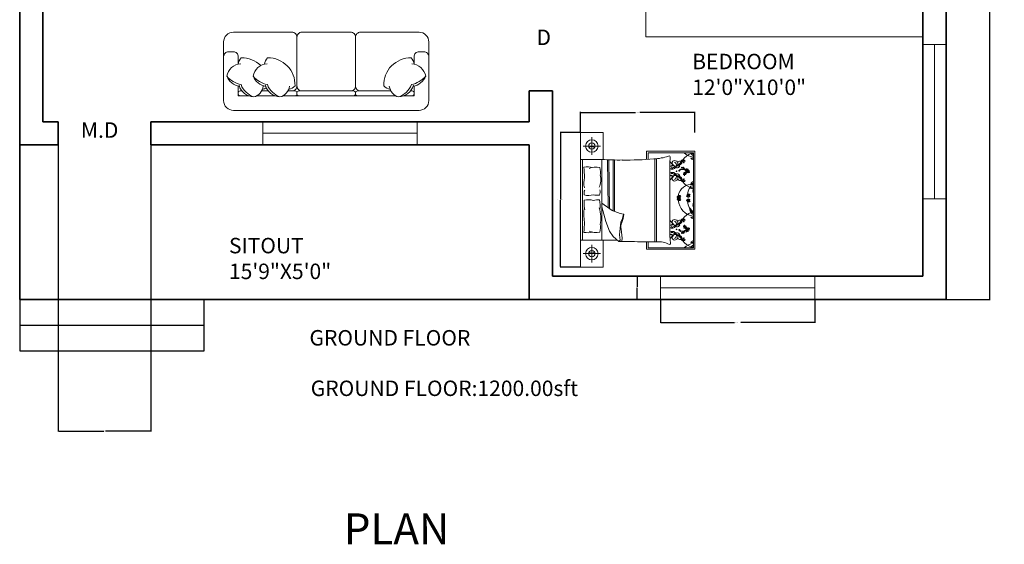
# Model space of a CAD drawing. Units: inches. Extents: x -43 to 1296, y -568 to 542.
# Tile 1 of 14: x 29 to 411, y -568 to -365. Entities that reach past the tile are written whole.
import ezdxf

# ---------------------------------------------------------------- set-up
doc = ezdxf.new("R2010")
doc.units = ezdxf.units.IN
doc.header["$MEASUREMENT"] = 0
for name, color, linetype, lineweight in [('A-ANNO-DIMS', 2, 'Continuous', 18), ('A-ANNO-TEXT', 7, 'Continuous', 18), ('A-AREA-IDEN', 7, 'Continuous', 18), ('A-FLOR-CASE', 9, 'Continuous', 18), ('A-FLOR-STRS', 7, 'Continuous', 25), ('A-FURN', 8, 'Continuous', 13), ('A-GLAZ', 6, 'Continuous', 18), ('A-WALL', 7, 'Continuous', 35)]:
    doc.layers.add(name, color=color, linetype=linetype, lineweight=lineweight)
doc.styles.get("Standard").update_dxf_attribs({"font": 'arial.ttf'})
doc.dimstyles.get("Standard").update_dxf_attribs({"dimtxt": 0.18, "dimasz": 0.18, "dimexe": 0.18, "dimexo": 0.0625, "dimgap": 0.09, "dimtad": 0, "dimtih": 1, "dimtoh": 1, "dimdec": 0, "dimzin": 0, "dimdsep": 46, "dimlunit": 3, "dimtxsty": 'Standard', "dimcen": 0.09, "dimadec": 0, "dimazin": 0, "dimtfac": 1, "dimtdec": 0, "dimtofl": 0, "dimtmove": 0, "dimatfit": 3, "dimfxl": 1, "dimtolj": 1, "dimtzin": 0, "dimarcsym": 0})

# ---------------------------------------------------------------- blocks, each defined once
blk = doc.blocks.new('*D2')
at = {"layer": 'A-ANNO-DIMS', "color": 0, "lineweight": -2, "transparency": 16777216}
for p, q in [((388.91, 6.66), (405.97, 6.66)), ((405.79, 6.48), (405.79, -230.19)), ((405.79, -473.16), (405.79, -236.49)), ((388.91, -473.34), (405.97, -473.34))]:
    blk.add_line(p, q, dxfattribs=at)
at = {"layer": 'A-ANNO-DIMS', "color": 0, "transparency": 16777216}
for points in [[(405.76, 6.48), (405.82, 6.48), (405.79, 6.66)], [(405.76, -473.16), (405.82, -473.16), (405.79, -473.34)]]:
    blk.add_solid(points, dxfattribs=at)
at = {"layer": 'Defpoints', "color": 0, "transparency": 16777216}
for p in [(388.84, 6.66), (388.84, -473.34), (405.79, -473.34)]:
    blk.add_point(p, dxfattribs=at)
at = {"layer": 'A-ANNO-DIMS', "color": 0, "transparency": 16777216, "insert": (405.79, -233.34), "char_height": 6, "attachment_point": 5}
blk.add_mtext("\\A1;40'", dxfattribs=at)
blk = doc.blocks.new('BED-SUITE-52')
for p, q in [((0, 0), (0, 52.23)), ((4.35, 43.59), (4.35, 50.42)), ((7.76, 47), (0.94, 47)), ((25.6, 42.07), (25.6, 44.97)), ((25.6, 44.97), (44.41, 44.97)), ((26.21, 44.36), (26.21, 42.06)), ((43.81, 44.36), (26.21, 44.36)), ((43.81, 7.5), (43.81, 44.36)), ((44.41, 44.97), (44.41, 6.89)), ((0.67, 41.78), (0.67, 10.45)), ((8.25, 10.45), (8.25, 41.78)), ((10.42, 41.64), (10.68, 23.05)), ((10.96, 41.62), (11.23, 22.66)), ((12.6, 41.59), (12.68, 21.76)), ((13.14, 41.6), (13.22, 21.56)), ((28.86, 42.02), (28.86, 9.84)), ((29.51, 42.07), (29.51, 9.84)), ((38.51, 39.22), (37.92, 39.33)), ((34.64, 36.72), (34.64, 15.51)), ((38.51, 35.57), (37.92, 35.45)), ((8.25, 24.79), (12.24, 21.93)), ((9.81, 17.7), (8.25, 23.4)), ((12.24, 21.93), (15.3, 20.77)), ((15.3, 20.77), (16.68, 20.56)), ((16.68, 20.56), (16.25, 18.86)), ((11.18, 13.89), (9.81, 17.7)), ((15.62, 17.49), (15.3, 15.16)), ((16.25, 18.86), (15.62, 17.49)), ((38.51, 16.3), (37.92, 16.41)), ((12.66, 11.88), (11.18, 13.89)), ((14.88, 9.98), (12.66, 11.88)), ((15.3, 15.16), (15.09, 12.52)), ((15.09, 12.52), (15.3, 10.4)), ((38.51, 12.65), (37.92, 12.53)), ((0, 10.45), (14.33, 10.45)), ((4.35, 8.64), (4.35, 1.81)), ((15.3, 10.4), (14.88, 9.98)), ((25.6, 6.89), (25.6, 9.85)), ((26.21, 9.85), (26.21, 7.5)), ((7.76, 5.22), (0.94, 5.22)), ((44.41, 6.89), (25.6, 6.89)), ((26.21, 7.5), (43.81, 7.5))]:
    blk.add_line(p, q)
for points in [[(0, 41.78), (8.7, 41.78), (8.7, 52.23), (0, 52.23)], [(4.35, 47), (3.3, 46.39)], [(4.35, 47), (5.41, 46.39)], [(8.7, 10.45), (8.7, 0), (0, 0)], [(4.35, 5.22), (3.3, 5.83)], [(4.35, 5.22), (5.41, 5.83)]]:
    blk.add_lwpolyline(points)
for points in [[(28.45, 42, 0.056112), (31.32, 42.38, 0.095341), (34.09, 43.12)], [(1.3, 38.78, -0.074897), (4.71, 38.72, 0.472817)], [(4.9, 28.1, -0.14099), (1.42, 27.99, -0.235245)], [(4.9, 25.87, 0.14099), (1.42, 25.97, 0.235245)], [(1.3, 13.45, 0.074897), (4.71, 13.51, -0.472817)], [(19.66, 9.87, 0.001242), (29.57, 9.84, -0.127202), (34.51, 8.8)]]:
    blk.add_lwpolyline(points, format="xyb")
for centre, radius in [((4.35, 47), 2.44), ((4.35, 47), 1.22), ((40.41, 36.2), 0.133), ((41.81, 37.07), 0.133), ((40.41, 15.66), 0.133), ((41.81, 14.79), 0.133), ((4.35, 5.22), 2.44), ((4.35, 5.22), 1.22)]:
    blk.add_circle(centre, radius)
for centre, radius, start, end in [((34.35, 42.72), 0.476, 336.5219, 123.8264), ((85.43, 38.32), 50.82, 175.2402, 181.8035), ((45.4, 37.77), 6.82, 111.4092, 145.6135), ((44.73, 49.44), 6.82, 228.1144, 262.255), ((45.64, 46.02), 3.32, 209.8884, 236.5383), ((44.87, 44.16), 2.77, 221.0454, 247.4453), ((43.38, 51.75), 9.44, 266.3481, 272.5919), ((46.26, 47.22), 4.14, 223.5186, 233.6964), ((-495.72, 9.99), 497.85, 2.8502, 3.3148), ((6.08, 32.13), 6.73, 78.2417, 114.8684), ((0.69, 36.92), 7, 348.9631, 14.8961), ((14.64, 135.41), 93.84, 266.1, 270.9282), ((18.05, 163.97), 122.41, 269.1145, 274.8735), ((35.22, 38.66), 0.629, 196.6343, 225.5483), ((35.03, 41.34), 2.16, 259.249, 301.1782), ((35.22, 38.66), 0.629, 127.675, 162.5814), ((38.32, 42.79), 3.95, 203.6453, 236.3329), ((35.59, 39.66), 1.66, 240.8249, 340.7178), ((35.09, 38.92), 0.781, 246.1646, 318.4347), ((35.97, 37.49), 2.01, 85.2696, 124.215), ((35.89, 39.91), 1.5, 240.0851, 262.564), ((36.42, 40.49), 0.882, 88.9462, 185.5144), ((37.07, 40.76), 1.57, 193.079, 274.7067), ((36.48, 37.7), 1.07, 74.8529, 138.4347), ((37.39, 39.86), 1.3, 196.8663, 330.0915), ((36.55, 40.12), 1.25, 7.1143, 95.0551), ((36.07, 39.63), 1.21, 338.5779, 68.4181), ((36.84, 39.04), 0.324, 254.8529, 12.6959), ((35.97, 37.49), 2.01, 53.6555, 57.2989), ((36.27, 40.34), 1.52, 305.9599, 357.6409), ((37.03, 41.99), 2.8, 273.4924, 303.7117), ((36.83, 41.97), 2.47, 288.2955, 328.7386), ((38.56, 40.41), 0.784, 19.1312, 189.736), ((38.32, 40.6), 0.979, 285.6955, 4.031), ((39.62, 39.55), 1.04, 128.4175, 173.8338), ((39.41, 40.57), 0.48, 126.7319, 206.0245), ((39.64, 41.08), 0.565, 76.272, 177.0484), ((38.78, 42.23), 1.16, 284.7031, 328.6173), ((39.25, 38.55), 0.103, 125.0752, 284.7644), ((39.41, 38.59), 0.222, 127.3642, 168.4363), ((39.24, 38.77), 0.32, 277.4968, 341.2737), ((40.4, 40.75), 1.08, 125.7657, 194.5347), ((35.12, 42.66), 4.77, 332.8176, 347.4827), ((39.49, 38.62), 0.127, 88.1325, 178.8919), ((39.75, 38.49), 0.275, 136.3462, 189.6513), ((39.62, 38.78), 0.133, 183.2768, 356.7232), ((39.59, 38.46), 0.115, 189.6513, 312.3208), ((40.03, 38.54), 0.435, 164.2829, 186.9148), ((39.52, 38.54), 0.218, 312.3208, 40.2111), ((39.98, 38.78), 0.309, 201.6382, 274.947), ((39.57, 38.36), 0.404, 42.3896, 66.5724), ((43.64, 41.56), 4.96, 217.9541, 226.8459), ((39.94, 40.89), 0.756, 20.9613, 102.2885), ((40.34, 41.64), 0.57, 181.7131, 301.5367), ((38.48, 40.49), 1.72, 2.0648, 41.1598), ((39.52, 41.13), 0.558, 316.2238, 62.3173), ((39.84, 40.8), 0.0445, 20.2667, 316.2271), ((39.86, 38.6), 0.22, 10.9597, 52.2379), ((40, 38.58), 0.102, 274.947, 37.5263), ((40.07, 40.56), 0.0411, 52.0591, 168.5166), ((40.11, 40.55), 0.0847, 168.5166, 2.0648), ((40.65, 38.13), 0.274, 115.5379, 168.6744), ((39.72, 38.52), 0.825, 329.344, 349.7412), ((39.06, 38.33), 1.47, 352.8698, 1.6736), ((10.44, 32.58), 9.18, 166.3427, 191.1841), ((1.21, 33.9), 6.65, 333.8761, 16.1746), ((35.22, 36.13), 0.629, 134.4517, 156.7144), ((35.22, 36.13), 0.629, 203.2856, 232.325), ((35.03, 33.45), 2.16, 58.8218, 100.2867), ((38.32, 32), 3.95, 123.6671, 158.5059), ((35.59, 35.12), 1.66, 19.2822, 119.1751), ((35.09, 35.86), 0.781, 41.5653, 113.8354), ((35.97, 37.29), 2.01, 235.785, 274.7304), ((35.89, 34.87), 1.5, 97.436, 119.9149), ((37.07, 34.03), 1.57, 85.2933, 166.921), ((36.48, 37.09), 1.07, 221.5653, 285.1471), ((37.39, 34.92), 1.3, 29.9085, 163.1337), ((36.55, 34.66), 1.25, 264.9449, 352.8857), ((36.07, 35.15), 1.21, 291.5819, 21.4221), ((36.84, 35.74), 0.324, 347.3041, 105.1471), ((35.97, 37.29), 2.01, 302.7011, 306.3445), ((37.27, 37.25), 0.164, 169.5864, 349.5616), ((36.27, 34.44), 1.52, 2.3591, 54.0401), ((37.03, 32.8), 2.8, 56.2883, 86.5076), ((37.33, 37.24), 0.101, 349.5616, 167.2949), ((36.83, 32.82), 2.47, 31.2614, 71.7045), ((38.56, 34.37), 0.784, 170.264, 340.8688), ((39.96, 33.62), 4.33, 110.1059, 116.9968), ((38.51, 37.19), 0.274, 129.5056, 182.6421), ((37.73, 37.82), 0.825, 308.4388, 328.836), ((37.58, 38.49), 1.47, 296.5064, 305.3102), ((37.57, 37.74), 0.839, 336.3901, 344.4871), ((38.48, 37.52), 0.106, 83.9457, 185.6216), ((38.06, 37.62), 0.438, 328.836, 0.8141), ((38.28, 37.49), 0.251, 306.5232, 32.4668), ((38.58, 37.69), 0.106, 112.5583, 214.2343), ((38.51, 37.88), 0.251, 265.7131, 351.6568), ((38.29, 38.02), 0.438, 297.3659, 329.344), ((37.96, 38.39), 0.839, 313.6929, 321.7899), ((39.62, 35.24), 1.04, 186.1662, 231.5825), ((38.32, 34.18), 0.979, 355.969, 74.3045), ((38.89, 37.82), 0.274, 115.5379, 168.6744), ((37.96, 38.21), 0.825, 329.344, 349.7412), ((39.96, 33.62), 4.33, 86.1723, 106.4158), ((37.3, 38.02), 1.47, 352.8698, 1.6736), ((40.04, 35.98), 0.103, 125.0752, 284.7644), ((40.2, 36.02), 0.222, 93.635, 168.4363), ((40.21, 37.22), 0.606, 253.6301, 325.4631), ((40.38, 36.38), 0.429, 82.0748, 142.6895), ((40.33, 36.97), 0.441, 228.342, 274.9894), ((40.17, 36.37), 0.13, 138.2946, 276.2474), ((40.03, 36.19), 0.32, 277.4968, 341.2737), ((40.22, 36.35), 0.181, 358.5719, 143.8954), ((40.28, 36.04), 0.127, 88.1325, 178.8919), ((40.33, 36.49), 0.183, 208.8493, 269.9355), ((40.17, 36.45), 0.209, 274.2123, 318.1587), ((40.34, 38), 0.106, 112.5583, 214.2343), ((40.27, 38.19), 0.251, 265.7131, 351.6568), ((40.05, 38.33), 0.438, 297.3659, 329.344), ((40.07, 35.78), 2.17, 60.7959, 85.244), ((35.46, 32.66), 7.14, 37.8256, 47.7588), ((40.54, 35.91), 0.275, 136.3462, 189.6513), ((40.38, 35.88), 0.115, 189.6513, 312.3208), ((39.72, 38.7), 0.839, 313.6929, 321.7899), ((42.95, 35.55), 2.6, 175.2415, 182.8929), ((40.34, 36.89), 0.369, 273.8774, 357.1501), ((40.82, 35.96), 0.435, 164.2829, 186.9148), ((40.81, 36.24), 0.419, 121.9501, 165.2442), ((40.49, 37.15), 0.357, 262.0748, 308.2393), ((40.31, 35.96), 0.218, 312.3208, 40.2111), ((40.77, 36.2), 0.309, 201.6382, 274.947), ((40.52, 36.4), 0.0881, 262.868, 7.094), ((40.36, 35.78), 0.404, 42.3896, 66.5724), ((40.51, 36.47), 0.262, 278.5614, 22.5914), ((40.65, 36.02), 0.22, 10.9597, 118.7804), ((42.95, 35.55), 2.6, 156.1523, 156.9499), ((40.66, 36.48), 0.132, 44.3732, 121.9501), ((41.06, 36.79), 0.369, 181.4625, 249.4747), ((42.95, 35.55), 2.6, 130.182, 149.456), ((41, 37.08), 0.357, 215.1128, 261.2773), ((41.29, 37.06), 0.606, 197.889, 269.722), ((40.79, 36), 0.102, 274.947, 37.5263), ((41.1, 36.85), 0.441, 248.3627, 295.0101), ((40.88, 36.3), 0.429, 20.6625, 81.2773), ((41.13, 38.04), 0.148, 33.0979, 123.1364), ((37.86, 35.94), 3.89, 31.1156, 34.8118), ((40.91, 37.78), 0.402, 2.3172, 70.5201), ((41.52, 37.04), 0.429, 139.3812, 199.9959), ((40.72, 37.35), 0.606, 310.9365, 22.7695), ((41, 37.31), 0.441, 285.6484, 332.2957), ((41.25, 37.68), 0.116, 135.7354, 318.1297), ((41.05, 37.87), 0.154, 315.7354, 31.1156), ((40.92, 37.55), 0.357, 319.3812, 5.5456), ((41.33, 37.68), 0.116, 68.2452, 250.6395), ((41.07, 37.83), 0.346, 352.6008, 57.1845), ((42.3, 35.5), 2.32, 111.7087, 116.2181), ((41.4, 37.91), 0.346, 252.8042, 349.6943), ((41.07, 37.29), 0.369, 331.1838, 51.6792), ((40.07, 35.78), 2.17, 47.5083, 55.9967), ((41.44, 36.85), 0.103, 125.0752, 284.7644), ((41.43, 37.93), 0.154, 248.2452, 323.6254), ((41.6, 36.89), 0.222, 93.635, 168.4363), ((41.57, 37.24), 0.13, 138.2946, 276.2474), ((41.3, 38.03), 0.402, 291.7087, 3.0299), ((41.43, 37.06), 0.32, 277.4968, 341.2737), ((41.62, 37.22), 0.181, 358.5719, 143.8954), ((38.43, 40.15), 3.89, 323.6254, 327.3216), ((41.68, 36.91), 0.127, 88.1325, 178.8919), ((41.73, 37.36), 0.183, 208.8493, 269.9355), ((41.57, 37.32), 0.209, 274.2123, 318.1587), ((41.94, 36.78), 0.275, 136.3462, 189.6513), ((41.78, 36.75), 0.115, 189.6513, 312.3208), ((41.61, 37.93), 0.148, 325.6077, 55.6462), ((42.22, 36.83), 0.435, 164.2829, 186.9148), ((42.21, 37.11), 0.419, 121.9501, 165.2442), ((41.71, 36.83), 0.218, 312.3208, 40.2111), ((42.17, 37.07), 0.309, 201.6382, 274.947), ((41.92, 37.27), 0.0881, 262.868, 7.094), ((41.76, 36.65), 0.404, 42.3896, 66.5724), ((41.91, 37.34), 0.262, 278.5614, 22.5914), ((42.06, 36.89), 0.22, 10.9597, 118.7804), ((42.06, 37.35), 0.132, 44.3732, 121.9501), ((42.19, 36.87), 0.102, 274.947, 37.5263), ((36.42, 34.3), 0.882, 174.4856, 271.0538), ((43.15, 26.86), 5.28, 82.8636, 171.8197), ((39.41, 34.21), 0.48, 153.9755, 233.2681), ((39.64, 33.71), 0.565, 182.9516, 283.728), ((38.78, 32.55), 1.16, 31.3827, 75.2969), ((40.4, 34.03), 1.08, 165.4653, 234.2343), ((35.12, 32.13), 4.77, 12.5173, 27.1824), ((38.48, 34.29), 1.72, 318.8402, 357.9352), ((39.52, 33.65), 0.558, 297.6827, 43.7762), ((40.34, 33.14), 0.57, 58.4633, 178.2869), ((39.94, 33.9), 0.756, 257.7115, 339.0387), ((45.4, 37.01), 6.82, 214.3865, 248.5908), ((39.86, 33.99), 0.0738, 43.7762, 339.7183), ((40.11, 34.24), 0.0847, 357.9352, 191.4834), ((40.07, 34.23), 0.0411, 191.4834, 307.9409), ((48.38, 27.61), 6.82, 152.5854, 175.5377), ((43.52, 30.35), 1.22, 76.3898, 169.0739), ((43.35, 29.43), 1.55, 72.8609, 131.9049), ((44.87, 30.63), 2.77, 112.5547, 138.9546), ((43.38, 23.03), 9.44, 87.4081, 93.6519), ((47.4, 29.51), 3.75, 162.9798, 196.4569), ((3.91, 28.71), 2.58, 153.3437, 196.1026), ((6.65, 34.26), 6.4, 254.1707, 275.9871), ((4.81, 29.06), 2.77, 335.0183, 18.5407), ((38.09, 27.07), 0.565, 106.1963, 206.9726), ((38.09, 26.53), 0.565, 153.0274, 253.8037), ((36.76, 27.64), 1.16, 314.6273, 358.5415), ((36.76, 25.96), 1.16, 1.4585, 45.3727), ((38.91, 27.17), 1.08, 155.6899, 224.4589), ((38.91, 26.43), 1.08, 135.5411, 204.3101), ((38.44, 27.05), 0.756, 50.8855, 132.2127), ((38.41, 27.91), 0.57, 211.6373, 331.4609), ((37.95, 27.06), 0.558, 346.148, 92.2415), ((37.37, 25.98), 1.72, 31.989, 71.0841), ((33.38, 26.19), 4.77, 2.7418, 17.407), ((33.38, 27.42), 4.77, 342.593, 357.2582), ((38.39, 26.93), 0.0445, 50.1909, 346.0209), ((38.76, 26.85), 0.0847, 198.4408, 31.989), ((38.72, 26.84), 0.0411, 81.9833, 198.4408), ((38.76, 26.75), 0.0847, 328.011, 161.5592), ((41.74, 27.59), 0.565, 106.1963, 206.9726), ((40.42, 28.17), 1.16, 314.6273, 358.5415), ((42.56, 27.69), 1.08, 155.6899, 224.4589), ((42.09, 27.58), 0.756, 50.8855, 132.2127), ((42.07, 28.44), 0.57, 211.6373, 331.4609), ((41.02, 26.51), 1.72, 31.989, 71.0841), ((37.03, 26.71), 4.77, 2.7418, 17.407), ((41.6, 27.58), 0.558, 346.148, 92.2415), ((42.05, 27.46), 0.0445, 50.1909, 346.0209), ((42.67, 27.55), 3.05, 68.117, 96.6195), ((42.41, 27.37), 0.0847, 198.4408, 31.989), ((42.37, 27.36), 0.0411, 81.9833, 198.4408), ((49.33, 28.03), 5.55, 174.3643, 175.6213), ((53.13, 25.11), 9.91, 160.0972, 160.2783), ((20.2, 20.6), 18.94, 172.2196, 189.497), ((10.63, 24.6), 9.31, 171.5249, 193.96), ((6.65, 19.71), 6.4, 84.0129, 105.8293), ((-4.28, 18.99), 12.14, 348.0397, 19.2615), ((-1.63, 23.91), 9.21, 349.8617, 13.6238), ((37.37, 27.62), 1.72, 288.9159, 328.011), ((37.95, 26.55), 0.558, 267.7585, 13.852), ((38.41, 25.69), 0.57, 28.5391, 148.3627), ((38.44, 26.55), 0.756, 227.7873, 309.1145), ((44.73, 26.52), 6.82, 184.4623, 262.255), ((38.42, 26.66), 0.0738, 13.852, 309.9245), ((38.72, 26.77), 0.0411, 161.5592, 278.0167), ((41.74, 26.01), 0.565, 153.0274, 253.8037), ((40.42, 25.44), 1.16, 1.4585, 45.3727), ((42.56, 25.91), 1.08, 135.5411, 204.3101), ((37.03, 26.89), 4.77, 342.593, 357.2582), ((41.02, 27.1), 1.72, 288.9159, 328.011), ((41.6, 26.02), 0.558, 267.7585, 13.852), ((42.07, 25.17), 0.57, 28.5391, 148.3627), ((42.09, 26.03), 0.756, 227.7873, 309.1145), ((48.38, 26), 6.82, 184.4623, 207.4146), ((42.07, 26.14), 0.0738, 13.852, 309.9245), ((45.64, 23.1), 3.32, 181.272, 236.5383), ((47.43, 26.47), 6.16, 214.0123, 234.053), ((46.26, 24.29), 4.14, 197.8504, 233.6964), ((42.41, 26.23), 0.0847, 328.011, 161.5592), ((42.37, 26.24), 0.0411, 161.5592, 278.0167), ((47.4, 24.09), 3.75, 163.5431, 197.0202), ((49.33, 25.58), 5.55, 184.3787, 185.6357), ((53.13, 28.5), 9.91, 199.7217, 199.9028), ((-3.06, 24.18), 20.25, 340.1194, 349.3383), ((16.72, 20.44), 0.126, 358.8623, 109.7536), ((45.4, 14.85), 6.82, 111.4092, 145.6135), ((43.38, 28.83), 9.44, 266.3481, 272.5919), ((44.87, 21.24), 2.77, 221.0454, 247.4453), ((-495.72, 42.23), 497.85, 356.6852, 357.1498), ((0.69, 15.31), 7, 345.1039, 11.0369), ((19.88, 15.58), 4.25, 156.2616, 191.3392), ((38.32, 19.87), 3.95, 201.4941, 236.3329), ((35.03, 18.42), 2.16, 259.7133, 301.1782), ((35.22, 15.74), 0.629, 127.675, 156.7144), ((89, 14.89), 54.37, 179.3433, 185.6887), ((35.22, 15.74), 0.629, 203.229, 225.5483), ((35.59, 16.74), 1.66, 240.8249, 340.7178), ((35.09, 16), 0.781, 246.1646, 318.4347), ((35.97, 14.57), 2.01, 85.2696, 124.215), ((35.89, 16.99), 1.5, 240.0851, 262.564), ((36.42, 17.56), 0.882, 88.9462, 185.5144), ((37.07, 17.84), 1.57, 193.079, 274.7067), ((36.48, 14.77), 1.07, 74.8529, 138.4347), ((37.39, 16.94), 1.3, 196.8663, 330.0915), ((36.55, 17.2), 1.25, 7.1143, 95.0551), ((36.07, 16.71), 1.21, 338.5779, 68.4181), ((36.84, 16.12), 0.324, 254.8529, 12.6959), ((35.97, 14.57), 2.01, 53.6555, 57.2989), ((36.27, 17.42), 1.52, 305.9599, 357.6409), ((37.03, 19.07), 2.8, 273.4924, 303.7117), ((36.83, 19.04), 2.47, 288.2955, 328.7386), ((38.56, 17.49), 0.784, 19.1312, 189.736), ((38.32, 17.68), 0.979, 285.6955, 4.031), ((39.62, 16.62), 1.04, 128.4175, 173.8338), ((39.41, 17.65), 0.48, 126.7319, 206.0245), ((39.64, 18.15), 0.565, 76.272, 177.0484), ((38.78, 19.31), 1.16, 284.7031, 328.6173), ((40.4, 17.83), 1.08, 125.7657, 194.5347), ((35.12, 19.74), 4.77, 332.8176, 347.4827), ((39.94, 17.96), 0.756, 20.9613, 102.2885), ((39.52, 18.21), 0.558, 316.2238, 62.3173), ((38.48, 17.57), 1.72, 2.0648, 41.1598), ((40.34, 18.72), 0.57, 181.7131, 301.5367), ((39.84, 17.88), 0.0445, 20.2667, 316.2271), ((40.04, 15.89), 0.103, 75.2356, 234.9248), ((40.2, 15.85), 0.222, 191.5637, 266.365), ((40.07, 17.64), 0.0411, 52.0591, 168.5166), ((40.11, 17.63), 0.0847, 168.5166, 2.0648), ((40.17, 15.5), 0.13, 83.7526, 221.7054), ((40.33, 14.9), 0.441, 85.0106, 131.658), ((40.03, 15.67), 0.32, 18.7263, 82.5032), ((40.22, 15.52), 0.181, 216.1046, 1.4281), ((40.28, 15.82), 0.127, 181.1081, 271.8675), ((40.33, 15.37), 0.183, 90.0645, 151.1507), ((40.17, 15.42), 0.209, 41.8413, 85.7877), ((40.54, 15.95), 0.275, 170.3487, 223.6538), ((40.38, 15.98), 0.115, 47.6792, 170.3487), ((42.95, 16.31), 2.6, 177.1071, 184.7585), ((40.34, 14.97), 0.369, 2.8499, 86.1226), ((40.82, 15.9), 0.435, 173.0852, 195.7171), ((40.81, 15.63), 0.419, 194.7558, 238.0499), ((40.31, 15.9), 0.218, 319.7889, 47.6792), ((40.77, 15.66), 0.309, 85.053, 158.3618), ((40.52, 15.47), 0.0881, 352.906, 97.132), ((40.36, 16.08), 0.404, 293.4276, 317.6104), ((40.65, 15.84), 0.22, 241.2196, 349.0403), ((40.51, 15.39), 0.262, 337.4086, 81.4386), ((41.06, 15.07), 0.369, 110.5253, 178.5375), ((41.29, 14.8), 0.606, 90.278, 162.111), ((40.79, 15.86), 0.102, 322.4737, 85.053), ((41.1, 15.01), 0.441, 64.9899, 111.6373), ((40.88, 15.56), 0.429, 278.7227, 339.3375), ((6.08, 20.1), 6.73, 245.1316, 281.7583), ((-3.62, 10.87), 19.71, 357.4519, 11.3392), ((35.22, 13.2), 0.629, 134.4517, 153.558), ((35.22, 13.2), 0.629, 210.0293, 232.325), ((35.03, 10.52), 2.16, 58.8218, 99.1554), ((35.59, 12.2), 1.66, 19.2822, 119.1751), ((35.09, 12.94), 0.781, 41.5653, 113.8354), ((38.32, 9.07), 3.95, 123.6671, 153.2997), ((35.97, 14.37), 2.01, 235.785, 274.7304), ((35.89, 11.95), 1.5, 97.436, 119.9149), ((37.07, 11.11), 1.57, 85.2933, 166.921), ((36.48, 14.17), 1.07, 221.5653, 285.1471), ((37.39, 12), 1.3, 29.9085, 163.1337), ((36.55, 11.74), 1.25, 264.9449, 352.8857), ((36.07, 12.23), 1.21, 291.5819, 21.4221), ((36.84, 12.82), 0.324, 347.3041, 105.1471), ((35.97, 14.37), 2.01, 302.7011, 306.3445), ((37.27, 14.61), 0.164, 10.4384, 190.4136), ((36.27, 11.52), 1.52, 2.3591, 54.0401), ((37.03, 9.87), 2.8, 56.2883, 86.5076), ((37.33, 14.62), 0.101, 192.7051, 10.4384), ((36.83, 9.9), 2.47, 31.2614, 71.7045), ((38.56, 11.45), 0.784, 170.264, 340.8688), ((39.96, 18.24), 4.33, 243.0032, 249.8941), ((37.73, 14.04), 0.825, 31.164, 51.5612), ((38.51, 14.68), 0.274, 177.3579, 230.4944), ((37.58, 13.37), 1.47, 54.6898, 63.4936), ((37.57, 14.13), 0.839, 15.5129, 23.6099), ((38.48, 14.34), 0.106, 174.3784, 276.0543), ((38.28, 14.37), 0.251, 327.5332, 53.4768), ((38.06, 14.24), 0.438, 359.1859, 31.164), ((38.58, 14.18), 0.106, 145.7657, 247.4417), ((38.51, 13.99), 0.251, 8.3432, 94.2869), ((38.29, 13.85), 0.438, 30.656, 62.6341), ((37.96, 13.47), 0.839, 38.2101, 46.3071), ((38.32, 11.26), 0.979, 355.969, 74.3045), ((39.62, 12.32), 1.04, 186.1662, 231.5825), ((38.89, 14.04), 0.274, 191.3256, 244.4621), ((37.96, 13.65), 0.825, 10.2588, 30.656), ((39.96, 18.24), 4.33, 253.5842, 273.8277), ((37.3, 13.84), 1.47, 358.3264, 7.1302), ((39.41, 11.29), 0.48, 153.9755, 233.2681), ((39.25, 13.31), 0.103, 75.2356, 234.9248), ((39.41, 13.27), 0.222, 191.5637, 232.6358), ((39.24, 13.09), 0.32, 18.7263, 82.5032), ((39.49, 13.24), 0.127, 181.1081, 271.8675), ((39.75, 13.37), 0.275, 170.3487, 223.6538), ((39.59, 13.4), 0.115, 47.6792, 170.3487), ((39.62, 13.08), 0.133, 3.2768, 176.7232), ((40.03, 13.32), 0.435, 173.0852, 195.7171), ((39.52, 13.33), 0.218, 319.7889, 47.6792), ((39.98, 13.08), 0.309, 85.053, 158.3618), ((43.64, 10.31), 4.96, 133.1541, 142.0459), ((39.57, 13.5), 0.404, 293.4276, 317.6104), ((39.86, 13.27), 0.22, 307.7621, 349.0403), ((40, 13.29), 0.102, 322.4737, 85.053), ((40.21, 14.64), 0.606, 34.5369, 106.3699), ((40.38, 15.49), 0.429, 217.3105, 277.9252), ((40.34, 13.86), 0.106, 145.7657, 247.4417), ((35.46, 19.21), 7.14, 312.2412, 322.1744), ((40.07, 16.09), 2.17, 274.756, 299.2041), ((40.27, 13.67), 0.251, 8.3432, 94.2869), ((40.05, 13.54), 0.438, 30.656, 62.6341), ((39.72, 13.16), 0.839, 38.2101, 46.3071), ((40.65, 13.73), 0.274, 191.3256, 244.4621), ((39.72, 13.34), 0.825, 10.2588, 30.656), ((40.49, 14.71), 0.357, 51.7607, 97.9252), ((39.06, 13.53), 1.47, 358.3264, 7.1302), ((42.95, 16.31), 2.6, 203.0501, 203.8477), ((40.66, 15.38), 0.132, 238.0499, 315.6268), ((41, 14.78), 0.357, 98.7227, 144.8872), ((42.95, 16.31), 2.6, 210.544, 229.818), ((40.91, 14.08), 0.402, 289.4799, 357.6828), ((37.86, 15.92), 3.89, 325.1882, 328.8844), ((41.13, 13.83), 0.148, 236.8636, 326.9021), ((41.52, 14.83), 0.429, 160.0041, 220.6188), ((40.72, 14.52), 0.606, 337.2305, 49.0635), ((41, 14.55), 0.441, 27.7043, 74.3516), ((41.25, 14.18), 0.116, 41.8703, 224.2646), ((41.05, 13.99), 0.154, 328.8844, 44.2646), ((40.92, 14.32), 0.357, 354.4544, 40.6188), ((41.33, 14.18), 0.116, 109.3605, 291.7548), ((41.07, 14.04), 0.346, 302.8155, 7.3992), ((42.3, 16.36), 2.32, 243.7819, 248.2913), ((41.07, 14.58), 0.369, 308.3208, 28.8162), ((40.07, 16.09), 2.17, 304.0033, 312.4917), ((41.4, 13.96), 0.346, 10.3057, 107.1958), ((41.44, 15.02), 0.103, 75.2356, 234.9248), ((41.43, 13.93), 0.154, 36.3746, 111.7548), ((41.6, 14.98), 0.222, 191.5637, 266.365), ((41.57, 14.63), 0.13, 83.7526, 221.7054), ((41.3, 13.83), 0.402, 356.9701, 68.2913), ((41.43, 14.8), 0.32, 18.7263, 82.5032), ((41.62, 14.65), 0.181, 216.1046, 1.4281), ((41.68, 14.95), 0.127, 181.1081, 271.8675), ((38.43, 11.71), 3.89, 32.6784, 36.3746), ((41.73, 14.5), 0.183, 90.0645, 151.1507), ((41.57, 14.55), 0.209, 41.8413, 85.7877), ((41.94, 15.08), 0.275, 170.3487, 223.6538), ((41.78, 15.11), 0.115, 47.6792, 170.3487), ((41.61, 13.94), 0.148, 304.3538, 34.3923), ((42.22, 15.03), 0.435, 173.0852, 195.7171), ((42.21, 14.76), 0.419, 194.7558, 238.0499), ((41.71, 15.03), 0.218, 319.7889, 47.6792), ((42.17, 14.79), 0.309, 85.053, 158.3618), ((41.92, 14.6), 0.0881, 352.906, 97.132), ((41.76, 15.21), 0.404, 293.4276, 317.6104), ((42.06, 14.97), 0.22, 241.2196, 349.0403), ((41.91, 14.52), 0.262, 337.4086, 81.4386), ((42.06, 14.51), 0.132, 238.0499, 315.6268), ((42.19, 14.99), 0.102, 322.4737, 85.053), ((16.18, -37.91), 47.9, 85.8294, 91.553), ((34.48, 9.28), 0.482, 273.98, 27.3412), ((36.42, 11.38), 0.882, 174.4856, 271.0538), ((38.78, 9.63), 1.16, 31.3827, 75.2969), ((39.64, 10.79), 0.565, 182.9516, 283.728), ((40.4, 11.11), 1.08, 165.4653, 234.2343), ((35.12, 9.2), 4.77, 12.5173, 27.1824), ((38.48, 11.37), 1.72, 318.8402, 357.9352), ((39.52, 10.73), 0.558, 297.6827, 43.7762), ((40.34, 10.22), 0.57, 58.4633, 178.2869), ((39.94, 10.98), 0.756, 257.7115, 339.0387), ((45.4, 14.09), 6.82, 214.3865, 248.5908), ((39.86, 11.07), 0.0738, 43.7762, 339.7183), ((40.11, 11.31), 0.0847, 357.9352, 191.4834), ((40.07, 11.31), 0.0411, 191.4834, 307.9409), ((44.73, 2.42), 6.82, 97.745, 131.8856), ((45.64, 5.84), 3.32, 123.4617, 150.1116), ((44.87, 7.7), 2.77, 112.5547, 138.9546), ((43.38, 0.11), 9.44, 87.4081, 93.6519), ((46.26, 4.65), 4.14, 126.3036, 136.4814)]:
    blk.add_arc(centre, radius, start, end)
blk = doc.blocks.new('WIN-60x9')
for p, q in [((0, 60), (0, 0)), ((9, 60), (0, 60)), ((4.5, 60), (4.5, 0)), ((9, 0), (9, 60)), ((0, 0), (9, 0))]:
    blk.add_line(p, q)
blk = doc.blocks.new('STEPS-SITOUT')
for p, q in [((0, 20), (0, 10)), ((71.73, 0), (71.73, 20)), ((0, 10), (0, 0)), ((0, 10), (71.73, 10)), ((0, 0), (71.73, 0))]:
    blk.add_line(p, q)
blk = doc.blocks.new('*D32')
at = {"layer": 'A-ANNO-DIMS', "color": 0, "lineweight": -2, "transparency": 16777216}
for p, q in [((277.84, -473.4), (277.84, -482.52)), ((337.84, -473.4), (337.84, -482.52)), ((278.02, -482.34), (306.61, -482.34)), ((337.66, -482.34), (309.07, -482.34))]:
    blk.add_line(p, q, dxfattribs=at)
at = {"layer": 'A-ANNO-DIMS', "color": 0, "transparency": 16777216}
for points in [[(278.02, -482.31), (278.02, -482.37), (277.84, -482.34)], [(337.66, -482.31), (337.66, -482.37), (337.84, -482.34)]]:
    blk.add_solid(points, dxfattribs=at)
at = {"layer": 'Defpoints', "color": 0, "transparency": 16777216}
for p in [(277.84, -473.34), (337.84, -473.34), (337.84, -482.34)]:
    blk.add_point(p, dxfattribs=at)
at = {"layer": 'A-ANNO-DIMS', "color": 0, "transparency": 16777216, "insert": (307.84, -482.34), "char_height": 0.18, "attachment_point": 5}
blk.add_mtext('\\A1;WINDOW 5\'-0" TYP.', dxfattribs=at)
blk = doc.blocks.new('*D33')
at = {"layer": 'A-ANNO-DIMS', "color": 0, "lineweight": -2, "transparency": 16777216}
for p, q in [((277.78, -464.34), (268.66, -464.34)), ((268.84, -464.52), (268.84, -468.66)), ((268.84, -473.16), (268.84, -469.02)), ((277.78, -473.34), (268.66, -473.34))]:
    blk.add_line(p, q, dxfattribs=at)
at = {"layer": 'A-ANNO-DIMS', "color": 0, "transparency": 16777216}
for points in [[(268.81, -464.52), (268.87, -464.52), (268.84, -464.34)], [(268.81, -473.16), (268.87, -473.16), (268.84, -473.34)]]:
    blk.add_solid(points, dxfattribs=at)
at = {"layer": 'Defpoints', "color": 0, "transparency": 16777216}
for p in [(277.84, -464.34), (268.84, -473.34), (277.84, -473.34)]:
    blk.add_point(p, dxfattribs=at)
at = {"layer": 'A-ANNO-DIMS', "color": 0, "transparency": 16777216, "insert": (268.84, -468.84), "char_height": 0.18, "attachment_point": 5}
blk.add_mtext('\\A1;0\'-9" TYP.', dxfattribs=at)
blk = doc.blocks.new('*D42')
at = {"layer": 'A-ANNO-DIMS', "color": 0, "lineweight": -2, "transparency": 16777216}
for p, q in [((246.76, -408.57), (238.81, -408.57)), ((238.99, -408.75), (238.99, -434.5)), ((238.99, -460.61), (238.99, -434.86)), ((246.76, -460.79), (238.81, -460.79))]:
    blk.add_line(p, q, dxfattribs=at)
at = {"layer": 'A-ANNO-DIMS', "color": 0, "transparency": 16777216}
for points in [[(238.96, -408.75), (239.02, -408.75), (238.99, -408.57)], [(238.96, -460.61), (239.02, -460.61), (238.99, -460.79)]]:
    blk.add_solid(points, dxfattribs=at)
at = {"layer": 'Defpoints', "color": 0, "transparency": 16777216}
for p in [(238.99, -408.57), (246.83, -408.57), (246.83, -460.79)]:
    blk.add_point(p, dxfattribs=at)
at = {"layer": 'A-ANNO-DIMS', "color": 0, "transparency": 16777216, "insert": (238.99, -434.68), "char_height": 0.18, "attachment_point": 5}
blk.add_mtext('\\A1;BED SET 4\'-4" TYP.', dxfattribs=at)
blk = doc.blocks.new('*D43')
at = {"layer": 'A-ANNO-DIMS', "color": 0, "lineweight": -2, "transparency": 16777216}
for p, q in [((246.83, -408.51), (246.83, -400.55)), ((247.01, -400.73), (268.19, -400.73)), ((291.06, -400.73), (269.88, -400.73)), ((291.24, -408.51), (291.24, -400.55))]:
    blk.add_line(p, q, dxfattribs=at)
at = {"layer": 'A-ANNO-DIMS', "color": 0, "transparency": 16777216}
for points in [[(247.01, -400.7), (247.01, -400.76), (246.83, -400.73)], [(291.06, -400.7), (291.06, -400.76), (291.24, -400.73)]]:
    blk.add_solid(points, dxfattribs=at)
at = {"layer": 'Defpoints', "color": 0, "transparency": 16777216}
for p in [(291.24, -400.73), (246.83, -408.57), (291.24, -408.57)]:
    blk.add_point(p, dxfattribs=at)
at = {"layer": 'A-ANNO-DIMS', "color": 0, "transparency": 16777216, "insert": (269.03, -400.73), "char_height": 0.18, "attachment_point": 5}
blk.add_mtext('\\A1;3\'-8 1/2" TYP.', dxfattribs=at)
blk = doc.blocks.new('*D58')
at = {"layer": 'A-ANNO-DIMS', "color": 0, "lineweight": -2, "transparency": 16777216}
for p, q in [((43.84, -413.4), (43.84, -524.67)), ((79.84, -413.4), (79.84, -524.67)), ((44.02, -524.49), (61.51, -524.49)), ((79.66, -524.49), (62.17, -524.49))]:
    blk.add_line(p, q, dxfattribs=at)
at = {"layer": 'A-ANNO-DIMS', "color": 0, "transparency": 16777216}
for points in [[(44.02, -524.46), (44.02, -524.52), (43.84, -524.49)], [(79.66, -524.46), (79.66, -524.52), (79.84, -524.49)]]:
    blk.add_solid(points, dxfattribs=at)
at = {"layer": 'Defpoints', "color": 0, "transparency": 16777216}
for p in [(43.84, -413.34), (79.84, -413.34), (79.84, -524.49)]:
    blk.add_point(p, dxfattribs=at)
at = {"layer": 'A-ANNO-DIMS', "color": 0, "transparency": 16777216, "insert": (61.84, -524.49), "char_height": 0.18, "attachment_point": 5}
blk.add_mtext('\\A1;3\'-0"', dxfattribs=at)

msp = doc.modelspace()

# ---------------------------------------------------------------- linework, layer by layer
at = {"layer": 'A-FLOR-CASE'}
for p, q in [((272.21, -344.34), (272.21, -371.34)), ((272.21, -371.34), (379.84, -371.34))]:
    msp.add_line(p, q, dxfattribs=at)
at = {"layer": 'A-FURN', "ltscale": 0.03}
msp.add_lwpolyline([(187.82, -373.39, 0.414214), (184.03, -369.59), (161.25, -369.59, 0.414214), (159.35, -371.49, 0.414214), (157.45, -369.59), (138.47, -369.59, 0.414214), (136.57, -371.49, 0.414214), (134.67, -369.59), (111.9, -369.59, 0.414214), (108.1, -373.39), (108.1, -396.17, 0.414214), (111.9, -399.96), (184.03, -399.96, 0.414214), (187.82, -396.17)], format="xyb", close=True, dxfattribs=at)
at = {"layer": 'A-FURN'}
for points in [[(134.67, -392.37, 0.414214), (136.57, -390.47), (136.57, -371.49, 0.414214)], [(161.25, -392.37, -0.414214), (159.35, -390.47), (159.35, -371.49, -0.414214)], [(113.79, -382.03), (113.79, -379.09, 0.414214), (111.9, -377.19), (110, -377.19, 0.414214), (108.1, -379.09)], [(187.82, -379.09, 0.414214), (185.92, -377.19), (184.03, -377.19, 0.414214), (182.13, -379.09), (182.13, -382.03)], [(114.75, -381.91, 0.356772), (109.31, -386.7, 0.249542), (114.24, -390.64, -9.61688)], [(113.79, -382.03, -0.165541), (114.96, -379.52, -0.200231), (122.5, -382.57, -0.121523)], [(124.97, -381.91, 0.356772), (119.53, -386.7, 0.249542), (124.46, -390.64, -9.61688)], [(124.02, -382.03, -0.165541), (125.19, -379.52, -0.425989), (135.85, -390.39, -0.121523), (133.32, -391.89, 7.115464)], [(182.13, -382.03, 0.165541), (180.96, -379.52, 0.425989), (170.3, -390.39, 0.121523), (172.83, -391.89, -7.115464)], [(181.17, -381.91, -0.356772), (186.61, -386.7, -0.249542), (181.69, -390.64, 9.61688)], [(109.31, -386.7, 0.14773), (114.86, -389.96, 0.213343), (119.75, -394.74, 0.178662)], [(114.09, -390.22, 0.306663), (119.75, -394.74, 0.30633), (123.45, -390.61, -0.872847)], [(119.53, -386.7, 0.14773), (125.08, -389.96, 0.213343), (129.98, -394.74, 0.178662)], [(124.31, -390.22, 0.306663), (129.98, -394.74, 0.30633), (133.67, -390.61, -0.872847)], [(181.83, -390.22, -0.306663), (176.17, -394.74, -0.30633), (172.47, -390.61, 0.872847)], [(186.61, -386.7, -0.14773), (181.07, -389.96, -0.213343), (176.17, -394.74, -0.178662)], [(117.79, -394.27), (113.79, -394.27), (113.79, -390.54, 0.414214)], [(115.24, -392.37), (114.55, -392.37, 0.414214), (113.79, -393.13), (113.79, -393.51, 0.414214), (114.55, -394.27)], [(125.47, -392.37), (122.86, -392.37, 0.414214)], [(124.69, -391.15, -0.071865), (123.09, -391.89, 7.115464)], [(131.17, -394.27), (135.81, -394.27, 0.414214), (136.57, -393.51), (136.57, -393.13, 0.414214), (135.81, -392.37), (133.08, -392.37, 0.414214)], [(138.47, -392.37, -0.414214), (136.57, -390.47)], [(157.45, -392.37, 0.414214), (159.35, -390.47)], [(174.98, -394.27), (160.11, -394.27, -0.414214), (159.35, -393.51), (159.35, -393.13, -0.414214), (160.11, -392.37), (173.06, -392.37, -0.414214)], [(180.68, -392.37), (181.37, -392.37, -0.414214), (182.13, -393.13), (182.13, -393.51, -0.414214), (181.37, -394.27)], [(114.55, -394.27), (117.79, -394.27, 0.414214)], [(120.95, -394.27), (128.01, -394.27, 0.414214)], [(181.37, -394.27), (178.13, -394.27, -0.414214)]]:
    msp.add_lwpolyline(points, format="xyb", dxfattribs=at)
msp.add_lwpolyline([(137.33, -394.27), (158.59, -394.27, 0.414214), (159.35, -393.51), (159.35, -393.13, 0.414214), (158.59, -392.37), (137.33, -392.37, 0.414214), (136.57, -393.13), (136.57, -393.51, 0.414214)], format="xyb", close=True, dxfattribs=at)
for points in [[(182.13, -390.54), (182.13, -394.27), (178.13, -394.27)], [(128.01, -394.27), (120.95, -394.27)], [(174.98, -394.27), (131.17, -394.27)]]:
    msp.add_lwpolyline(points, dxfattribs=at)
at = {"layer": 'A-WALL'}
for p, q in [((28.84, 6.66), (28.84, -473.34)), ((388.84, 6.66), (388.84, -473.34)), ((37.84, -260.34), (37.84, -404.34)), ((379.84, -344.34), (379.84, -464.34)), ((226.84, -392.34), (235.84, -392.34)), ((226.84, -392.34), (226.84, -404.34)), ((235.84, -392.34), (235.84, -464.34)), ((37.84, -404.34), (43.84, -404.34)), ((43.84, -404.34), (43.84, -413.34)), ((79.84, -413.34), (79.84, -404.34)), ((79.84, -404.34), (226.84, -404.34)), ((28.84, -413.34), (43.84, -413.34)), ((79.84, -413.34), (226.84, -413.34)), ((226.84, -413.34), (226.84, -473.34)), ((235.84, -464.34), (379.84, -464.34)), ((28.84, -473.34), (388.84, -473.34))]:
    msp.add_line(p, q, dxfattribs=at)

# ---------------------------------------------------------------- block references
at = {"layer": 'A-FLOR-STRS'}
msp.add_blockref('STEPS-SITOUT', (28.84, -493.34), dxfattribs=at)
at = {"layer": 'A-FURN'}
msp.add_blockref('BED-SUITE-52', (246.83, -460.8), dxfattribs=at)
at = {"layer": 'A-GLAZ'}
msp.add_blockref('WIN-60x9', (379.84, -434.34), dxfattribs=at)
for p, rotation in [((123.34, -404.34), 270.0000000000003), ((277.84, -464.34), 270.0000000000002)]:
    msp.add_blockref('WIN-60x9', p, dxfattribs=dict(at, rotation=rotation))

# ---------------------------------------------------------------- texts
at = {"layer": 'A-ANNO-TEXT', "attachment_point": 1}
for s, insert, char_height in [('D', (229.67, -368.58), 6), ('M.D', (52.64, -404.6), 6), ('GROUND FLOOR', (141.46, -485.27), 6), ('PLAN', (154.79, -556.47), 12)]:
    msp.add_mtext(s, dxfattribs=dict(at, insert=insert, char_height=char_height))
at = {"layer": 'A-AREA-IDEN', "char_height": 6, "attachment_point": 1}
for s, insert in [('BEDROOM\\P12\'0"X10\'0"', (290.18, -377.97)), ('SITOUT\\P15\'9"X5\'0"', (110.17, -449.47))]:
    msp.add_mtext(s, dxfattribs=dict(at, insert=insert))
at = {"layer": 'A-AREA-IDEN', "insert": (141.95, -504.89), "char_height": 6, "attachment_point": 1}
msp.add_mtext_dynamic_manual_height_columns('GROUND FLOOR:1200.00sft', width=119.732, gutter_width=1, heights=[15.32], dxfattribs=at)

# ---------------------------------------------------------------- dimensions: what is measured, and where the dimension line sits
at = {"layer": 'A-ANNO-DIMS'}
dim = msp.add_linear_dim(base=(405.79, -473.34), p1=(388.84, 6.66), p2=(388.84, -473.34), angle=90, dimstyle='Standard', override={"dimtxt": 6, "dimclrd": 0, "dimclre": 0, "dimclrt": 0}, dxfattribs=at)
dim.commit()
dim.dimension.update_dxf_attribs({"geometry": '*D2', "text_midpoint": (405.79, -233.34)})
dim = msp.add_linear_dim(base=(291.24, -400.73), p1=(246.83, -408.57), p2=(291.24, -408.57), text='<> TYP.', dimstyle='Standard', override={"dimdec": 1, "dimlfac": 1, "dimrnd": 0, "dimzin": 1, "dimdsep": 46, "dimlunit": 4, "dimfrac": 2}, dxfattribs=at)
dim.commit()
dim.dimension.update_dxf_attribs({"geometry": '*D43', "text_midpoint": (269.03, -400.73)})
for base, p1, p2, angle, text, picture, middle in [((238.99, -408.57), (246.83, -460.79), (246.83, -408.57), 90, 'BED SET <> TYP.', '*D42', (238.99, -434.68)), ((268.84, -473.34), (277.84, -464.34), (277.84, -473.34), 270, '<> TYP.', '*D33', (268.84, -468.84)), ((337.84, -482.34), (277.84, -473.34), (337.84, -473.34), 0, 'WINDOW <> TYP.', '*D32', (307.84, -482.34))]:
    dim = msp.add_linear_dim(base=base, p1=p1, p2=p2, angle=angle, text=text, dimstyle='Standard', override={"dimdec": 1, "dimlfac": 1, "dimrnd": 0, "dimzin": 1, "dimdsep": 46, "dimlunit": 4, "dimfrac": 2}, dxfattribs=at)
    dim.commit()
    dim.dimension.update_dxf_attribs({"geometry": picture, "text_midpoint": middle})
dim = msp.add_linear_dim(base=(79.84, -524.49), p1=(43.84, -413.34), p2=(79.84, -413.34), dimstyle='Standard', override={"dimdec": 1, "dimlfac": 1, "dimrnd": 0, "dimzin": 1, "dimdsep": 46, "dimlunit": 4, "dimfrac": 2}, dxfattribs=at)
dim.commit()
dim.dimension.update_dxf_attribs({"geometry": '*D58', "text_midpoint": (61.84, -524.49)})

doc.saveas('drawing.dxf')
